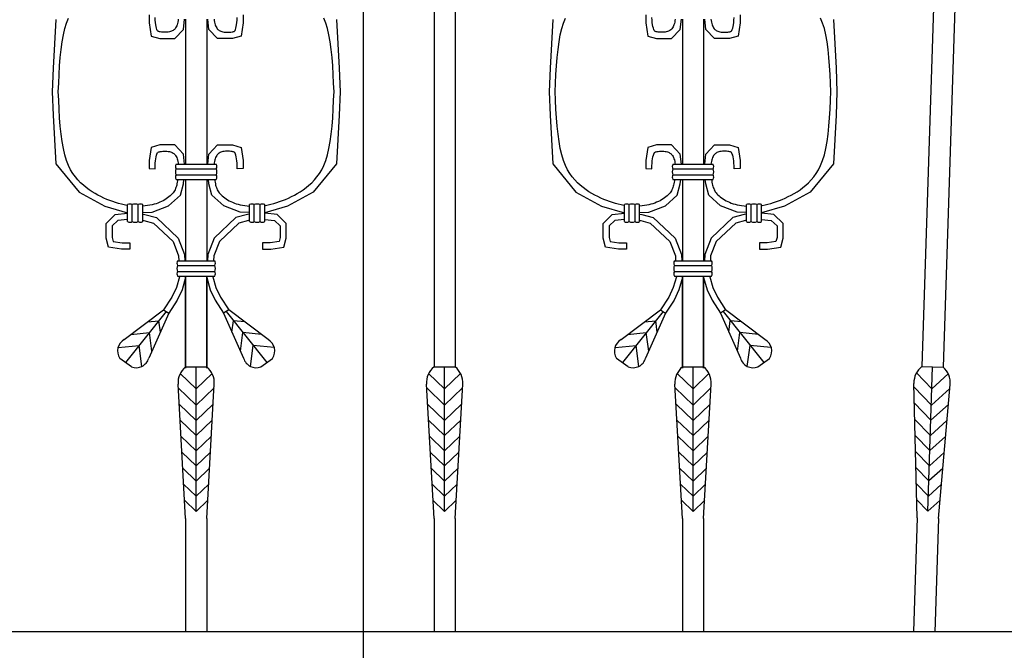
# Model space of a CAD drawing. Units: inches. Extents: x 2278 to 7495, y -71 to 1198.
# Tile 19 of 44: x 5007 to 5033, y 126 to 143. Entities that reach past the tile are written whole.
import ezdxf

# ---------------------------------------------------------------- set-up
doc = ezdxf.new("R2010")
doc.units = ezdxf.units.IN
doc.header["$MEASUREMENT"] = 0
doc.layers.add('A-ANNO-DIMS', color=2, linetype='Continuous', lineweight=18)
doc.layers.add('A-ELEV', color=7, linetype='Continuous', lineweight=25)
doc.styles.get("Standard").update_dxf_attribs({"font": 'arial.ttf'})
doc.dimstyles.get("Standard").update_dxf_attribs({"dimtxt": 6, "dimasz": 3, "dimexe": 0.18, "dimexo": 0.0625, "dimgap": 0.09, "dimtad": 0, "dimtih": 1, "dimtoh": 1, "dimdec": 0, "dimzin": 0, "dimdsep": 46, "dimlunit": 3, "dimtxsty": 'Standard', "dimblk": 'ARCHTICK', "dimcen": 0.09, "dimadec": 0, "dimazin": 0, "dimtfac": 1, "dimtdec": 0, "dimtofl": 0, "dimtmove": 0, "dimatfit": 3, "dimfxl": 1, "dimtolj": 1, "dimtzin": 0, "dimarcsym": 0})

# ---------------------------------------------------------------- blocks, each defined once
blk = doc.blocks.new('BALUSTER-ORNATE-A')
for p, q in [((0.096, 16.469), (0.025, 15.162)), ((0.386, 16.376), (0.438, 16.508)), ((2.602, 16.596), (2.602, 16.378)), ((2.769, 16.452), (2.766, 16.522)), ((2.775, 16.388), (2.769, 16.452)), ((3.383, 16.441), (3.376, 16.401)), ((3.388, 16.479), (3.383, 16.441)), ((3.528, 16.206), (3.557, 16.479)), ((3.585, 16.479), (3.585, 12.578)), ((4.155, 16.479), (4.155, 12.578)), ((4.212, 16.206), (4.183, 16.479)), ((4.352, 16.479), (4.357, 16.441)), ((4.357, 16.441), (4.364, 16.401)), ((4.965, 16.388), (4.971, 16.452)), ((4.971, 16.452), (4.974, 16.522)), ((5.138, 16.596), (5.138, 16.378)), ((7.354, 16.376), (7.302, 16.508)), ((7.644, 16.469), (7.715, 15.162)), ((0.3, 16.057), (0.34, 16.227)), ((0.34, 16.227), (0.386, 16.376)), ((2.602, 16.378), (2.656, 16.024)), ((2.783, 16.331), (2.775, 16.388)), ((2.792, 16.28), (2.783, 16.331)), ((2.803, 16.237), (2.792, 16.28)), ((2.815, 16.203), (2.803, 16.237)), ((2.825, 16.18), (2.815, 16.203)), ((2.834, 16.166), (2.825, 16.18)), ((2.84, 16.159), (2.834, 16.166)), ((2.846, 16.154), (2.84, 16.159)), ((2.852, 16.151), (2.846, 16.154)), ((3.205, 16.154), (3.179, 16.145)), ((3.228, 16.164), (3.205, 16.154)), ((3.249, 16.176), (3.228, 16.164)), ((3.268, 16.19), (3.249, 16.176)), ((3.286, 16.207), (3.268, 16.19)), ((3.303, 16.225), (3.286, 16.207)), ((3.292, 15.961), (3.528, 16.206)), ((3.318, 16.247), (3.303, 16.225)), ((3.333, 16.271), (3.318, 16.247)), ((3.346, 16.299), (3.333, 16.271)), ((3.357, 16.329), (3.346, 16.299)), ((3.368, 16.364), (3.357, 16.329)), ((3.376, 16.401), (3.368, 16.364)), ((4.448, 15.961), (4.212, 16.206)), ((4.364, 16.401), (4.372, 16.364)), ((4.372, 16.364), (4.383, 16.329)), ((4.383, 16.329), (4.394, 16.299)), ((4.394, 16.299), (4.407, 16.271)), ((4.407, 16.271), (4.422, 16.247)), ((4.422, 16.247), (4.437, 16.225)), ((4.437, 16.225), (4.454, 16.207)), ((4.454, 16.207), (4.472, 16.19)), ((4.472, 16.19), (4.491, 16.176)), ((4.491, 16.176), (4.512, 16.164)), ((4.512, 16.164), (4.535, 16.154)), ((4.535, 16.154), (4.561, 16.145)), ((4.888, 16.151), (4.895, 16.154)), ((4.895, 16.154), (4.9, 16.159)), ((4.9, 16.159), (4.906, 16.166)), ((4.906, 16.166), (4.915, 16.18)), ((4.915, 16.18), (4.925, 16.203)), ((4.925, 16.203), (4.937, 16.237)), ((4.937, 16.237), (4.948, 16.28)), ((4.948, 16.28), (4.957, 16.331)), ((4.957, 16.331), (4.965, 16.388)), ((5.138, 16.378), (5.084, 16.024)), ((7.4, 16.227), (7.354, 16.376)), ((7.44, 16.057), (7.4, 16.227)), ((0.267, 15.87), (0.3, 16.057)), ((2.656, 16.024), (2.892, 15.961)), ((2.863, 16.146), (2.852, 16.151)), ((2.88, 16.142), (2.863, 16.146)), ((2.905, 16.137), (2.88, 16.142)), ((2.892, 15.961), (3.292, 15.961)), ((2.936, 16.134), (2.905, 16.137)), ((2.971, 16.131), (2.936, 16.134)), ((3.008, 16.129), (2.971, 16.131)), ((3.045, 16.129), (3.008, 16.129)), ((3.081, 16.13), (3.045, 16.129)), ((3.117, 16.133), (3.081, 16.13)), ((3.15, 16.138), (3.117, 16.133)), ((3.179, 16.145), (3.15, 16.138)), ((4.848, 15.961), (4.448, 15.961)), ((4.561, 16.145), (4.59, 16.138)), ((4.59, 16.138), (4.623, 16.133)), ((4.623, 16.133), (4.659, 16.13)), ((4.659, 16.13), (4.695, 16.129)), ((4.695, 16.129), (4.732, 16.129)), ((4.732, 16.129), (4.769, 16.131)), ((4.769, 16.131), (4.804, 16.134)), ((4.804, 16.134), (4.835, 16.137)), ((4.835, 16.137), (4.86, 16.142)), ((5.084, 16.024), (4.848, 15.961)), ((4.86, 16.142), (4.877, 16.146)), ((4.877, 16.146), (4.888, 16.151)), ((7.473, 15.87), (7.44, 16.057)), ((0.217, 15.452), (0.239, 15.667)), ((0.239, 15.667), (0.267, 15.87)), ((7.501, 15.667), (7.473, 15.87)), ((7.523, 15.452), (7.501, 15.667)), ((0.199, 15.227), (0.217, 15.452)), ((7.541, 15.227), (7.523, 15.452)), ((0.025, 15.162), (0, 14.529)), ((0.185, 14.995), (0.199, 15.227)), ((7.555, 14.995), (7.541, 15.227)), ((7.715, 15.162), (7.74, 14.529)), ((0.173, 14.759), (0.185, 14.995)), ((7.567, 14.759), (7.555, 14.995)), ((0.163, 14.522), (0.173, 14.759)), ((7.577, 14.522), (7.567, 14.759)), ((0, 14.529), (0.025, 13.895)), ((0.173, 14.298), (0.163, 14.536)), ((0.185, 14.062), (0.173, 14.298)), ((7.555, 14.062), (7.567, 14.298)), ((7.567, 14.298), (7.577, 14.536)), ((7.74, 14.529), (7.715, 13.895)), ((0.199, 13.831), (0.185, 14.062)), ((7.541, 13.831), (7.555, 14.062)), ((0.025, 13.895), (0.096, 12.589)), ((0.217, 13.606), (0.199, 13.831)), ((7.523, 13.606), (7.541, 13.831)), ((7.715, 13.895), (7.644, 12.589)), ((0.239, 13.391), (0.217, 13.606)), ((7.501, 13.391), (7.523, 13.606)), ((0.267, 13.188), (0.239, 13.391)), ((7.473, 13.188), (7.501, 13.391)), ((0.3, 13), (0.267, 13.188)), ((0.34, 12.831), (0.3, 13)), ((2.656, 13.033), (2.602, 12.679)), ((2.892, 13.097), (2.656, 13.033)), ((3.292, 13.097), (2.892, 13.097)), ((3.528, 12.852), (3.292, 13.097)), ((4.212, 12.852), (4.448, 13.097)), ((4.448, 13.097), (4.848, 13.097)), ((4.848, 13.097), (5.084, 13.033)), ((5.084, 13.033), (5.138, 12.679)), ((7.4, 12.831), (7.44, 13)), ((7.44, 13), (7.473, 13.188)), ((0.386, 12.681), (0.34, 12.831)), ((2.775, 12.669), (2.783, 12.727)), ((2.783, 12.727), (2.792, 12.778)), ((2.792, 12.778), (2.803, 12.82)), ((2.803, 12.82), (2.815, 12.854)), ((2.815, 12.854), (2.825, 12.878)), ((2.825, 12.878), (2.834, 12.892)), ((2.834, 12.892), (2.84, 12.899)), ((2.84, 12.899), (2.846, 12.903)), ((2.846, 12.903), (2.852, 12.907)), ((2.852, 12.907), (2.863, 12.911)), ((2.863, 12.911), (2.88, 12.916)), ((2.88, 12.916), (2.905, 12.92)), ((2.905, 12.92), (2.936, 12.924)), ((2.936, 12.924), (2.971, 12.927)), ((2.971, 12.927), (3.008, 12.929)), ((3.008, 12.929), (3.045, 12.929)), ((3.045, 12.929), (3.081, 12.928)), ((3.081, 12.928), (3.117, 12.924)), ((3.117, 12.924), (3.15, 12.919)), ((3.15, 12.919), (3.179, 12.912)), ((3.179, 12.912), (3.205, 12.904)), ((3.205, 12.904), (3.228, 12.893)), ((3.228, 12.893), (3.249, 12.881)), ((3.249, 12.881), (3.268, 12.867)), ((3.268, 12.867), (3.286, 12.851)), ((3.286, 12.851), (3.303, 12.832)), ((3.303, 12.832), (3.318, 12.811)), ((3.318, 12.811), (3.333, 12.786)), ((3.333, 12.786), (3.346, 12.759)), ((3.346, 12.759), (3.357, 12.728)), ((3.357, 12.728), (3.368, 12.694)), ((3.557, 12.578), (3.528, 12.852)), ((4.183, 12.578), (4.212, 12.852)), ((4.383, 12.728), (4.372, 12.694)), ((4.394, 12.759), (4.383, 12.728)), ((4.407, 12.786), (4.394, 12.759)), ((4.422, 12.811), (4.407, 12.786)), ((4.437, 12.832), (4.422, 12.811)), ((4.454, 12.851), (4.437, 12.832)), ((4.472, 12.867), (4.454, 12.851)), ((4.491, 12.881), (4.472, 12.867)), ((4.512, 12.893), (4.491, 12.881)), ((4.535, 12.904), (4.512, 12.893)), ((4.561, 12.912), (4.535, 12.904)), ((4.59, 12.919), (4.561, 12.912)), ((4.623, 12.924), (4.59, 12.919)), ((4.659, 12.928), (4.623, 12.924)), ((4.695, 12.929), (4.659, 12.928)), ((4.732, 12.929), (4.695, 12.929)), ((4.769, 12.927), (4.732, 12.929)), ((4.804, 12.924), (4.769, 12.927)), ((4.835, 12.92), (4.804, 12.924)), ((4.86, 12.916), (4.835, 12.92)), ((4.877, 12.911), (4.86, 12.916)), ((4.888, 12.907), (4.877, 12.911)), ((4.895, 12.903), (4.888, 12.907)), ((4.9, 12.899), (4.895, 12.903)), ((4.906, 12.892), (4.9, 12.899)), ((4.915, 12.878), (4.906, 12.892)), ((4.925, 12.854), (4.915, 12.878)), ((4.937, 12.82), (4.925, 12.854)), ((4.948, 12.778), (4.937, 12.82)), ((4.957, 12.727), (4.948, 12.778)), ((4.965, 12.669), (4.957, 12.727)), ((7.354, 12.681), (7.4, 12.831)), ((0.096, 12.589), (0.722, 11.827)), ((0.438, 12.549), (0.386, 12.681)), ((0.495, 12.433), (0.438, 12.549)), ((2.602, 12.679), (2.602, 12.462)), ((2.602, 12.462), (2.764, 12.459)), ((2.764, 12.459), (2.766, 12.536)), ((2.766, 12.536), (2.769, 12.605)), ((2.769, 12.605), (2.775, 12.669)), ((3.329, 12.578), (4.411, 12.578)), ((3.329, 12.456), (4.411, 12.456)), ((3.368, 12.694), (3.376, 12.656)), ((3.376, 12.656), (3.383, 12.616)), ((3.383, 12.616), (3.388, 12.578)), ((4.357, 12.616), (4.352, 12.578)), ((4.364, 12.656), (4.357, 12.616)), ((4.372, 12.694), (4.364, 12.656)), ((4.971, 12.605), (4.965, 12.669)), ((4.974, 12.536), (4.971, 12.605)), ((4.976, 12.459), (4.974, 12.536)), ((5.138, 12.462), (4.976, 12.459)), ((5.138, 12.679), (5.138, 12.462)), ((7.644, 12.589), (7.018, 11.827)), ((7.245, 12.433), (7.302, 12.549)), ((7.302, 12.549), (7.354, 12.681)), ((0.557, 12.33), (0.495, 12.433)), ((0.623, 12.239), (0.557, 12.33)), ((0.692, 12.157), (0.623, 12.239)), ((3.329, 12.293), (4.411, 12.293)), ((7.048, 12.157), (7.117, 12.239)), ((7.117, 12.239), (7.183, 12.33)), ((7.183, 12.33), (7.245, 12.433)), ((0.764, 12.083), (0.692, 12.157)), ((0.839, 12.015), (0.764, 12.083)), ((0.916, 11.952), (0.839, 12.015)), ((0.993, 11.894), (0.916, 11.952)), ((3.316, 11.924), (3.303, 11.895)), ((3.327, 11.954), (3.316, 11.924)), ((3.337, 11.986), (3.327, 11.954)), ((3.329, 12.171), (4.411, 12.171)), ((3.346, 12.02), (3.337, 11.986)), ((3.354, 12.056), (3.346, 12.02)), ((3.361, 12.095), (3.354, 12.056)), ((3.368, 12.136), (3.361, 12.095)), ((3.374, 12.171), (3.368, 12.136)), ((3.446, 11.745), (3.528, 12.053)), ((3.528, 12.053), (3.542, 12.171)), ((3.585, 12.171), (3.585, 9.98)), ((4.155, 12.171), (4.155, 9.98)), ((4.212, 12.053), (4.198, 12.171)), ((4.294, 11.745), (4.212, 12.053)), ((4.366, 12.171), (4.372, 12.136)), ((4.372, 12.136), (4.379, 12.095)), ((4.379, 12.095), (4.386, 12.056)), ((4.386, 12.056), (4.394, 12.02)), ((4.394, 12.02), (4.403, 11.986)), ((4.403, 11.986), (4.413, 11.954)), ((4.413, 11.954), (4.424, 11.924)), ((4.424, 11.924), (4.437, 11.895)), ((6.747, 11.894), (6.824, 11.952)), ((6.824, 11.952), (6.901, 12.015)), ((6.901, 12.015), (6.976, 12.083)), ((6.976, 12.083), (7.048, 12.157)), ((0.722, 11.827), (1.412, 11.455)), ((1.071, 11.841), (0.993, 11.894)), ((1.15, 11.793), (1.071, 11.841)), ((1.23, 11.748), (1.15, 11.793)), ((1.309, 11.708), (1.23, 11.748)), ((1.389, 11.67), (1.309, 11.708)), ((1.469, 11.635), (1.389, 11.67)), ((3.102, 11.673), (3.064, 11.647)), ((3.138, 11.701), (3.102, 11.673)), ((3.128, 11.464), (3.446, 11.745)), ((3.171, 11.729), (3.138, 11.701)), ((3.201, 11.757), (3.171, 11.729)), ((3.228, 11.785), (3.201, 11.757)), ((3.252, 11.813), (3.228, 11.785)), ((3.272, 11.841), (3.252, 11.813)), ((3.288, 11.868), (3.272, 11.841)), ((3.303, 11.895), (3.288, 11.868)), ((4.612, 11.464), (4.294, 11.745)), ((4.437, 11.895), (4.452, 11.868)), ((4.452, 11.868), (4.468, 11.841)), ((4.468, 11.841), (4.489, 11.813)), ((4.489, 11.813), (4.512, 11.785)), ((4.512, 11.785), (4.539, 11.757)), ((4.539, 11.757), (4.569, 11.729)), ((4.569, 11.729), (4.602, 11.701)), ((4.602, 11.701), (4.638, 11.673)), ((4.638, 11.673), (4.676, 11.647)), ((6.271, 11.635), (6.351, 11.67)), ((7.018, 11.827), (6.328, 11.455)), ((6.351, 11.67), (6.431, 11.708)), ((6.431, 11.708), (6.51, 11.748)), ((6.51, 11.748), (6.59, 11.793)), ((6.59, 11.793), (6.669, 11.841)), ((6.669, 11.841), (6.747, 11.894)), ((1.412, 11.455), (2.026, 11.276)), ((1.549, 11.603), (1.469, 11.635)), ((1.627, 11.574), (1.549, 11.603)), ((1.705, 11.548), (1.627, 11.574)), ((1.782, 11.524), (1.705, 11.548)), ((1.858, 11.504), (1.782, 11.524)), ((1.933, 11.487), (1.858, 11.504)), ((2.007, 11.473), (1.933, 11.487)), ((2.026, 11.47), (2.007, 11.473)), ((2.026, 11.037), (2.026, 11.493)), ((2.148, 11.037), (2.148, 11.493)), ((2.311, 11.037), (2.311, 11.493)), ((2.434, 11.037), (2.434, 11.493)), ((2.499, 11.457), (2.434, 11.451)), ((2.563, 11.465), (2.499, 11.457)), ((2.624, 11.476), (2.563, 11.465)), ((2.683, 11.488), (2.624, 11.476)), ((2.739, 11.502), (2.683, 11.488)), ((2.683, 11.291), (3.128, 11.464)), ((2.792, 11.518), (2.739, 11.502)), ((2.843, 11.535), (2.792, 11.518)), ((2.891, 11.555), (2.843, 11.535)), ((2.937, 11.576), (2.891, 11.555)), ((2.981, 11.598), (2.937, 11.576)), ((3.024, 11.622), (2.981, 11.598)), ((3.064, 11.647), (3.024, 11.622)), ((5.057, 11.291), (4.612, 11.464)), ((4.676, 11.647), (4.716, 11.622)), ((4.716, 11.622), (4.759, 11.598)), ((4.759, 11.598), (4.803, 11.576)), ((4.803, 11.576), (4.849, 11.555)), ((4.849, 11.555), (4.897, 11.535)), ((4.897, 11.535), (4.948, 11.518)), ((4.948, 11.518), (5.001, 11.502)), ((5.001, 11.502), (5.057, 11.488)), ((5.057, 11.488), (5.116, 11.476)), ((5.116, 11.476), (5.177, 11.465)), ((5.177, 11.465), (5.241, 11.457)), ((5.241, 11.457), (5.306, 11.451)), ((5.306, 11.037), (5.306, 11.493)), ((5.429, 11.037), (5.429, 11.493)), ((5.592, 11.037), (5.592, 11.493)), ((5.714, 11.037), (5.714, 11.493)), ((5.714, 11.47), (5.733, 11.473)), ((6.328, 11.455), (5.714, 11.276)), ((5.733, 11.473), (5.807, 11.487)), ((5.807, 11.487), (5.882, 11.504)), ((5.882, 11.504), (5.958, 11.524)), ((5.958, 11.524), (6.035, 11.548)), ((6.035, 11.548), (6.113, 11.574)), ((6.113, 11.574), (6.191, 11.603)), ((6.191, 11.603), (6.271, 11.635)), ((1.449, 10.988), (1.694, 11.225)), ((1.694, 11.225), (2.026, 11.261)), ((2.434, 11.28), (2.683, 11.291)), ((2.434, 11.232), (2.492, 11.225)), ((2.492, 11.225), (2.801, 11.143)), ((2.801, 11.143), (3.385, 10.594)), ((4.939, 11.143), (4.355, 10.594)), ((5.248, 11.225), (4.939, 11.143)), ((5.306, 11.28), (5.057, 11.291)), ((5.306, 11.232), (5.248, 11.225)), ((6.046, 11.225), (5.714, 11.261)), ((6.291, 10.988), (6.046, 11.225)), ((1.449, 10.589), (1.449, 10.988)), ((1.767, 11.069), (1.612, 10.919)), ((1.612, 10.919), (1.612, 10.611)), ((2.026, 11.097), (1.767, 11.069)), ((2.434, 11.067), (2.462, 11.064)), ((2.462, 11.064), (2.719, 10.996)), ((2.719, 10.996), (3.247, 10.501)), ((5.021, 10.996), (4.493, 10.501)), ((5.278, 11.064), (5.021, 10.996)), ((5.306, 11.067), (5.278, 11.064)), ((5.714, 11.097), (5.973, 11.069)), ((5.973, 11.069), (6.128, 10.919)), ((6.128, 10.919), (6.128, 10.611)), ((6.291, 10.589), (6.291, 10.988)), ((1.612, 10.611), (1.642, 10.498)), ((3.385, 10.594), (3.558, 10.149)), ((4.355, 10.594), (4.182, 10.149)), ((6.128, 10.611), (6.098, 10.498)), ((1.513, 10.353), (1.449, 10.589)), ((1.866, 10.298), (1.513, 10.353)), ((1.642, 10.498), (1.879, 10.461)), ((1.879, 10.461), (2.084, 10.461)), ((2.084, 10.461), (2.084, 10.298)), ((3.247, 10.501), (3.396, 10.115)), ((4.493, 10.501), (4.344, 10.115)), ((5.861, 10.461), (5.656, 10.461)), ((5.656, 10.461), (5.656, 10.298)), ((6.098, 10.498), (5.861, 10.461)), ((5.874, 10.298), (6.227, 10.353)), ((6.227, 10.353), (6.291, 10.589)), ((2.084, 10.298), (1.866, 10.298)), ((3.396, 10.115), (3.402, 9.98)), ((3.558, 10.149), (3.565, 9.98)), ((4.182, 10.149), (4.175, 9.98)), ((4.344, 10.115), (4.338, 9.98)), ((5.656, 10.298), (5.874, 10.298)), ((3.37, 9.98), (4.37, 9.98)), ((3.37, 9.858), (4.37, 9.858)), ((3.421, 9.552), (3.337, 9.262)), ((3.37, 9.695), (4.37, 9.695)), ((3.37, 9.573), (4.37, 9.573)), ((3.42, 9.573), (3.421, 9.552)), ((3.585, 9.532), (3.49, 9.205)), ((3.583, 9.573), (3.585, 9.532)), ((3.585, 9.573), (3.585, 7.095)), ((3.585, 7.095), (3.585, 9.573)), ((4.155, 9.573), (4.155, 7.095)), ((4.155, 7.095), (4.155, 9.573)), ((4.157, 9.573), (4.155, 9.532)), ((4.155, 9.532), (4.25, 9.205)), ((4.32, 9.573), (4.319, 9.552)), ((4.319, 9.552), (4.403, 9.262)), ((3.337, 9.262), (3.217, 9.001)), ((3.49, 9.205), (3.36, 8.922)), ((4.25, 9.205), (4.38, 8.922)), ((4.403, 9.262), (4.523, 9.001)), ((3.217, 9.001), (2.995, 8.66)), ((3.36, 8.922), (3.131, 8.571)), ((4.38, 8.922), (4.609, 8.571)), ((4.523, 9.001), (4.745, 8.66)), ((1.936, 7.866), (2.995, 8.66)), ((3.063, 8.615), (1.97, 7.244)), ((3.131, 8.571), (2.594, 7.362)), ((2.995, 8.66), (3.131, 8.571)), ((4.745, 8.66), (4.609, 8.571)), ((4.609, 8.571), (5.146, 7.362)), ((4.677, 8.615), (5.77, 7.244)), ((5.804, 7.866), (4.745, 8.66)), ((2.562, 8.34), (2.868, 8.37)), ((2.907, 8.066), (2.868, 8.37)), ((4.833, 8.066), (4.872, 8.37)), ((5.178, 8.34), (4.872, 8.37)), ((2.111, 8.002), (2.613, 8.051)), ((2.678, 7.551), (2.613, 8.051)), ((5.062, 7.551), (5.127, 8.051)), ((5.629, 8.002), (5.127, 8.051)), ((1.774, 7.651), (2.339, 7.706)), ((2.412, 7.143), (2.339, 7.706)), ((5.328, 7.143), (5.401, 7.706)), ((5.966, 7.651), (5.401, 7.706)), ((2.128, 7.128), (1.813, 7.359)), ((5.612, 7.128), (5.927, 7.359)), ((3.442, 6.952), (3.87, 6.538)), ((3.585, 7.128), (4.155, 7.128)), ((3.87, 3.24), (3.87, 7.128)), ((4.299, 6.952), (3.87, 6.538)), ((3.585, 3.055), (3.383, 6.664)), ((4.155, 3.055), (4.357, 6.664)), ((3.388, 6.562), (3.87, 6.097)), ((4.352, 6.562), (3.87, 6.097)), ((3.413, 6.131), (3.87, 5.689)), ((4.327, 6.131), (3.87, 5.689)), ((3.437, 5.699), (3.87, 5.28)), ((4.303, 5.699), (3.87, 5.28)), ((3.461, 5.268), (3.87, 4.872)), ((4.279, 5.268), (3.87, 4.872)), ((3.485, 4.836), (3.87, 4.464)), ((4.255, 4.836), (3.87, 4.464)), ((3.509, 4.405), (3.87, 4.056)), ((4.231, 4.405), (3.87, 4.056)), ((3.533, 3.973), (3.87, 3.648)), ((4.207, 3.973), (3.87, 3.648)), ((3.558, 3.542), (3.87, 3.24)), ((4.182, 3.542), (3.87, 3.24)), ((3.585, 3.055), (3.585, 0)), ((4.155, 3.055), (4.155, 0))]:
    blk.add_line(p, q)
for centre, radius, start, end in [((3.434, 12.517), 0.121, 149.7768, 210.2232), ((3.522, 12.375), 0.209, 157.1017, 202.8983), ((4.306, 12.517), 0.121, 329.7768, 30.2232), ((4.218, 12.375), 0.209, 337.1017, 22.8983), ((3.434, 12.232), 0.121, 149.7768, 210.2232), ((4.306, 12.232), 0.121, 329.7768, 30.2232), ((2.087, 11.388), 0.121, 59.7768, 120.2232), ((2.23, 11.3), 0.209, 67.1017, 112.8983), ((2.373, 11.388), 0.121, 59.7768, 120.2232), ((5.368, 11.388), 0.121, 59.7768, 120.2232), ((5.51, 11.3), 0.209, 67.1017, 112.8983), ((5.653, 11.388), 0.121, 59.7768, 120.2232), ((2.087, 11.142), 0.121, 239.7768, 300.2232), ((2.23, 11.23), 0.209, 247.1017, 292.8983), ((2.373, 11.142), 0.121, 239.7768, 300.2232), ((5.368, 11.142), 0.121, 239.7768, 300.2232), ((5.51, 11.23), 0.209, 247.1017, 292.8983), ((5.653, 11.142), 0.121, 239.7768, 300.2232), ((3.475, 9.919), 0.121, 149.7768, 210.2232), ((3.563, 9.776), 0.209, 157.1017, 202.8983), ((4.265, 9.919), 0.121, 329.7768, 30.2232), ((4.177, 9.776), 0.209, 337.1017, 22.8983), ((3.475, 9.634), 0.121, 149.7768, 210.2232), ((4.265, 9.634), 0.121, 329.7768, 30.2232), ((2.111, 7.555), 0.356, 119.3212, 213.425), ((5.629, 7.555), 0.356, 326.575, 60.6788), ((2.253, 7.462), 0.356, 249.4937, 343.5975), ((5.487, 7.462), 0.356, 196.4025, 290.5063), ((3.929, 6.703), 0.547, 128.9283, 183.9822), ((3.811, 6.703), 0.547, 356.0178, 51.0717)]:
    blk.add_arc(centre, radius, start, end)
blk = doc.blocks.new('BALUSTER-ORNATE-B')
for p, q in [((0.096, 16.469), (0.025, 15.162)), ((0.386, 16.376), (0.438, 16.508)), ((2.602, 16.596), (2.602, 16.378)), ((2.769, 16.452), (2.766, 16.522)), ((2.775, 16.388), (2.769, 16.452)), ((3.384, 16.441), (3.377, 16.401)), ((3.388, 16.479), (3.384, 16.441)), ((3.528, 16.206), (3.558, 16.479)), ((3.585, 16.479), (3.585, 12.578)), ((4.155, 16.479), (4.155, 12.578)), ((4.213, 16.206), (4.183, 16.479)), ((4.352, 16.479), (4.357, 16.441)), ((4.357, 16.441), (4.364, 16.401)), ((4.965, 16.388), (4.971, 16.452)), ((4.971, 16.452), (4.975, 16.522)), ((5.139, 16.596), (5.139, 16.378)), ((7.354, 16.376), (7.302, 16.508)), ((7.645, 16.469), (7.715, 15.162)), ((0.3, 16.057), (0.34, 16.227)), ((0.34, 16.227), (0.386, 16.376)), ((2.602, 16.378), (2.656, 16.024)), ((2.783, 16.331), (2.775, 16.388)), ((2.793, 16.28), (2.783, 16.331)), ((2.803, 16.237), (2.793, 16.28)), ((2.815, 16.203), (2.803, 16.237)), ((2.826, 16.18), (2.815, 16.203)), ((2.834, 16.166), (2.826, 16.18)), ((2.841, 16.159), (2.834, 16.166)), ((2.846, 16.154), (2.841, 16.159)), ((2.852, 16.151), (2.846, 16.154)), ((3.206, 16.154), (3.18, 16.145)), ((3.229, 16.164), (3.206, 16.154)), ((3.249, 16.176), (3.229, 16.164)), ((3.269, 16.19), (3.249, 16.176)), ((3.286, 16.207), (3.269, 16.19)), ((3.303, 16.225), (3.286, 16.207)), ((3.292, 15.961), (3.528, 16.206)), ((3.319, 16.247), (3.303, 16.225)), ((3.333, 16.271), (3.319, 16.247)), ((3.346, 16.299), (3.333, 16.271)), ((3.358, 16.329), (3.346, 16.299)), ((3.368, 16.364), (3.358, 16.329)), ((3.377, 16.401), (3.368, 16.364)), ((4.449, 15.961), (4.213, 16.206)), ((4.364, 16.401), (4.373, 16.364)), ((4.373, 16.364), (4.383, 16.329)), ((4.383, 16.329), (4.394, 16.299)), ((4.394, 16.299), (4.407, 16.271)), ((4.407, 16.271), (4.422, 16.247)), ((4.422, 16.247), (4.437, 16.225)), ((4.437, 16.225), (4.454, 16.207)), ((4.454, 16.207), (4.472, 16.19)), ((4.472, 16.19), (4.491, 16.176)), ((4.491, 16.176), (4.512, 16.164)), ((4.512, 16.164), (4.535, 16.154)), ((4.535, 16.154), (4.561, 16.145)), ((4.888, 16.151), (4.895, 16.154)), ((4.895, 16.154), (4.9, 16.159)), ((4.9, 16.159), (4.906, 16.166)), ((4.906, 16.166), (4.915, 16.18)), ((4.915, 16.18), (4.926, 16.203)), ((4.926, 16.203), (4.937, 16.237)), ((4.937, 16.237), (4.948, 16.28)), ((4.948, 16.28), (4.958, 16.331)), ((4.958, 16.331), (4.965, 16.388)), ((5.139, 16.378), (5.084, 16.024)), ((7.401, 16.227), (7.354, 16.376)), ((7.44, 16.057), (7.401, 16.227)), ((0.267, 15.87), (0.3, 16.057)), ((2.656, 16.024), (2.892, 15.961)), ((2.863, 16.146), (2.852, 16.151)), ((2.881, 16.142), (2.863, 16.146)), ((2.905, 16.137), (2.881, 16.142)), ((2.892, 15.961), (3.292, 15.961)), ((2.936, 16.134), (2.905, 16.137)), ((2.971, 16.131), (2.936, 16.134)), ((3.008, 16.129), (2.971, 16.131)), ((3.045, 16.129), (3.008, 16.129)), ((3.082, 16.13), (3.045, 16.129)), ((3.117, 16.133), (3.082, 16.13)), ((3.15, 16.138), (3.117, 16.133)), ((3.18, 16.145), (3.15, 16.138)), ((4.848, 15.961), (4.449, 15.961)), ((4.561, 16.145), (4.591, 16.138)), ((4.591, 16.138), (4.624, 16.133)), ((4.624, 16.133), (4.659, 16.13)), ((4.659, 16.13), (4.696, 16.129)), ((4.696, 16.129), (4.733, 16.129)), ((4.733, 16.129), (4.769, 16.131)), ((4.769, 16.131), (4.805, 16.134)), ((4.805, 16.134), (4.836, 16.137)), ((4.836, 16.137), (4.86, 16.142)), ((5.084, 16.024), (4.848, 15.961)), ((4.86, 16.142), (4.877, 16.146)), ((4.877, 16.146), (4.888, 16.151)), ((7.473, 15.87), (7.44, 16.057)), ((0.217, 15.452), (0.24, 15.667)), ((0.24, 15.667), (0.267, 15.87)), ((7.501, 15.667), (7.473, 15.87)), ((7.523, 15.452), (7.501, 15.667)), ((0.199, 15.227), (0.217, 15.452)), ((7.541, 15.227), (7.523, 15.452)), ((0.025, 15.162), (0, 14.529)), ((0.185, 14.995), (0.199, 15.227)), ((7.556, 14.995), (7.541, 15.227)), ((7.715, 15.162), (7.74, 14.529)), ((0.173, 14.759), (0.185, 14.995)), ((7.567, 14.759), (7.556, 14.995)), ((0.163, 14.522), (0.173, 14.759)), ((7.577, 14.522), (7.567, 14.759)), ((0, 14.529), (0.025, 13.895)), ((0.173, 14.298), (0.163, 14.536)), ((0.185, 14.062), (0.173, 14.298)), ((7.556, 14.062), (7.567, 14.298)), ((7.567, 14.298), (7.577, 14.536)), ((7.74, 14.529), (7.715, 13.895)), ((0.199, 13.831), (0.185, 14.062)), ((7.541, 13.831), (7.556, 14.062)), ((0.025, 13.895), (0.096, 12.589)), ((0.217, 13.606), (0.199, 13.831)), ((7.523, 13.606), (7.541, 13.831)), ((7.715, 13.895), (7.645, 12.589)), ((0.24, 13.391), (0.217, 13.606)), ((7.501, 13.391), (7.523, 13.606)), ((0.267, 13.188), (0.24, 13.391)), ((7.473, 13.188), (7.501, 13.391)), ((0.3, 13), (0.267, 13.188)), ((0.34, 12.831), (0.3, 13)), ((2.656, 13.033), (2.602, 12.679)), ((2.892, 13.097), (2.656, 13.033)), ((3.292, 13.097), (2.892, 13.097)), ((3.528, 12.852), (3.292, 13.097)), ((4.213, 12.852), (4.449, 13.097)), ((4.449, 13.097), (4.848, 13.097)), ((4.848, 13.097), (5.084, 13.033)), ((5.084, 13.033), (5.139, 12.679)), ((7.401, 12.831), (7.44, 13)), ((7.44, 13), (7.473, 13.188)), ((0.386, 12.681), (0.34, 12.831)), ((2.775, 12.669), (2.783, 12.727)), ((2.783, 12.727), (2.793, 12.778)), ((2.793, 12.778), (2.803, 12.82)), ((2.803, 12.82), (2.815, 12.854)), ((2.815, 12.854), (2.826, 12.878)), ((2.826, 12.878), (2.834, 12.892)), ((2.834, 12.892), (2.841, 12.899)), ((2.841, 12.899), (2.846, 12.903)), ((2.846, 12.903), (2.852, 12.907)), ((2.852, 12.907), (2.863, 12.911)), ((2.863, 12.911), (2.881, 12.916)), ((2.881, 12.916), (2.905, 12.92)), ((2.905, 12.92), (2.936, 12.924)), ((2.936, 12.924), (2.971, 12.927)), ((2.971, 12.927), (3.008, 12.929)), ((3.008, 12.929), (3.045, 12.929)), ((3.045, 12.929), (3.082, 12.928)), ((3.082, 12.928), (3.117, 12.924)), ((3.117, 12.924), (3.15, 12.919)), ((3.15, 12.919), (3.18, 12.912)), ((3.18, 12.912), (3.206, 12.904)), ((3.206, 12.904), (3.229, 12.893)), ((3.229, 12.893), (3.249, 12.881)), ((3.249, 12.881), (3.269, 12.867)), ((3.269, 12.867), (3.286, 12.851)), ((3.286, 12.851), (3.303, 12.832)), ((3.303, 12.832), (3.319, 12.811)), ((3.319, 12.811), (3.333, 12.786)), ((3.333, 12.786), (3.346, 12.759)), ((3.346, 12.759), (3.358, 12.728)), ((3.358, 12.728), (3.368, 12.694)), ((3.558, 12.578), (3.528, 12.852)), ((4.183, 12.578), (4.213, 12.852)), ((4.383, 12.728), (4.373, 12.694)), ((4.394, 12.759), (4.383, 12.728)), ((4.407, 12.786), (4.394, 12.759)), ((4.422, 12.811), (4.407, 12.786)), ((4.437, 12.832), (4.422, 12.811)), ((4.454, 12.851), (4.437, 12.832)), ((4.472, 12.867), (4.454, 12.851)), ((4.491, 12.881), (4.472, 12.867)), ((4.512, 12.893), (4.491, 12.881)), ((4.535, 12.904), (4.512, 12.893)), ((4.561, 12.912), (4.535, 12.904)), ((4.591, 12.919), (4.561, 12.912)), ((4.624, 12.924), (4.591, 12.919)), ((4.659, 12.928), (4.624, 12.924)), ((4.696, 12.929), (4.659, 12.928)), ((4.733, 12.929), (4.696, 12.929)), ((4.769, 12.927), (4.733, 12.929)), ((4.805, 12.924), (4.769, 12.927)), ((4.836, 12.92), (4.805, 12.924)), ((4.86, 12.916), (4.836, 12.92)), ((4.877, 12.911), (4.86, 12.916)), ((4.888, 12.907), (4.877, 12.911)), ((4.895, 12.903), (4.888, 12.907)), ((4.9, 12.899), (4.895, 12.903)), ((4.906, 12.892), (4.9, 12.899)), ((4.915, 12.878), (4.906, 12.892)), ((4.926, 12.854), (4.915, 12.878)), ((4.937, 12.82), (4.926, 12.854)), ((4.948, 12.778), (4.937, 12.82)), ((4.958, 12.727), (4.948, 12.778)), ((4.965, 12.669), (4.958, 12.727)), ((7.354, 12.681), (7.401, 12.831)), ((0.096, 12.589), (0.722, 11.827)), ((0.438, 12.549), (0.386, 12.681)), ((0.496, 12.433), (0.438, 12.549)), ((2.602, 12.679), (2.602, 12.462)), ((2.602, 12.462), (2.765, 12.459)), ((2.765, 12.459), (2.766, 12.536)), ((2.766, 12.536), (2.769, 12.605)), ((2.769, 12.605), (2.775, 12.669)), ((3.33, 12.578), (4.411, 12.578)), ((3.33, 12.456), (4.411, 12.456)), ((3.368, 12.694), (3.377, 12.656)), ((3.377, 12.656), (3.384, 12.616)), ((3.384, 12.616), (3.388, 12.578)), ((4.357, 12.616), (4.352, 12.578)), ((4.364, 12.656), (4.357, 12.616)), ((4.373, 12.694), (4.364, 12.656)), ((4.971, 12.605), (4.965, 12.669)), ((4.975, 12.536), (4.971, 12.605)), ((4.976, 12.459), (4.975, 12.536)), ((5.139, 12.462), (4.976, 12.459)), ((5.139, 12.679), (5.139, 12.462)), ((7.645, 12.589), (7.018, 11.827)), ((7.245, 12.433), (7.302, 12.549)), ((7.302, 12.549), (7.354, 12.681)), ((0.557, 12.33), (0.496, 12.433)), ((0.623, 12.239), (0.557, 12.33)), ((0.692, 12.157), (0.623, 12.239)), ((3.33, 12.293), (4.411, 12.293)), ((7.048, 12.157), (7.117, 12.239)), ((7.117, 12.239), (7.183, 12.33)), ((7.183, 12.33), (7.245, 12.433)), ((0.765, 12.083), (0.692, 12.157)), ((0.839, 12.015), (0.765, 12.083)), ((0.916, 11.952), (0.839, 12.015)), ((0.994, 11.894), (0.916, 11.952)), ((3.316, 11.924), (3.303, 11.895)), ((3.327, 11.954), (3.316, 11.924)), ((3.337, 11.986), (3.327, 11.954)), ((3.33, 12.171), (4.411, 12.171)), ((3.346, 12.02), (3.337, 11.986)), ((3.354, 12.056), (3.346, 12.02)), ((3.362, 12.095), (3.354, 12.056)), ((3.369, 12.136), (3.362, 12.095)), ((3.374, 12.171), (3.369, 12.136)), ((3.446, 11.745), (3.528, 12.053)), ((3.528, 12.053), (3.542, 12.171)), ((3.585, 12.171), (3.585, 9.98)), ((4.155, 12.171), (4.155, 9.98)), ((4.213, 12.053), (4.199, 12.171)), ((4.294, 11.745), (4.213, 12.053)), ((4.366, 12.171), (4.372, 12.136)), ((4.372, 12.136), (4.379, 12.095)), ((4.379, 12.095), (4.387, 12.056)), ((4.387, 12.056), (4.395, 12.02)), ((4.395, 12.02), (4.404, 11.986)), ((4.404, 11.986), (4.413, 11.954)), ((4.413, 11.954), (4.425, 11.924)), ((4.425, 11.924), (4.437, 11.895)), ((6.747, 11.894), (6.825, 11.952)), ((6.825, 11.952), (6.901, 12.015)), ((6.901, 12.015), (6.976, 12.083)), ((6.976, 12.083), (7.048, 12.157)), ((0.722, 11.827), (1.412, 11.455)), ((1.072, 11.841), (0.994, 11.894)), ((1.151, 11.793), (1.072, 11.841)), ((1.23, 11.748), (1.151, 11.793)), ((1.309, 11.708), (1.23, 11.748)), ((1.389, 11.67), (1.309, 11.708)), ((1.469, 11.635), (1.389, 11.67)), ((3.103, 11.673), (3.064, 11.647)), ((3.138, 11.701), (3.103, 11.673)), ((3.128, 11.464), (3.446, 11.745)), ((3.171, 11.729), (3.138, 11.701)), ((3.201, 11.757), (3.171, 11.729)), ((3.228, 11.785), (3.201, 11.757)), ((3.252, 11.813), (3.228, 11.785)), ((3.272, 11.841), (3.252, 11.813)), ((3.289, 11.868), (3.272, 11.841)), ((3.303, 11.895), (3.289, 11.868)), ((4.612, 11.464), (4.294, 11.745)), ((4.437, 11.895), (4.452, 11.868)), ((4.452, 11.868), (4.469, 11.841)), ((4.469, 11.841), (4.489, 11.813)), ((4.489, 11.813), (4.512, 11.785)), ((4.512, 11.785), (4.539, 11.757)), ((4.539, 11.757), (4.569, 11.729)), ((4.569, 11.729), (4.602, 11.701)), ((4.602, 11.701), (4.638, 11.673)), ((4.638, 11.673), (4.676, 11.647)), ((6.271, 11.635), (6.351, 11.67)), ((7.018, 11.827), (6.328, 11.455)), ((6.351, 11.67), (6.431, 11.708)), ((6.431, 11.708), (6.511, 11.748)), ((6.511, 11.748), (6.59, 11.793)), ((6.59, 11.793), (6.669, 11.841)), ((6.669, 11.841), (6.747, 11.894)), ((1.412, 11.455), (2.027, 11.276)), ((1.549, 11.603), (1.469, 11.635)), ((1.628, 11.574), (1.549, 11.603)), ((1.705, 11.548), (1.628, 11.574)), ((1.782, 11.524), (1.705, 11.548)), ((1.858, 11.504), (1.782, 11.524)), ((1.933, 11.487), (1.858, 11.504)), ((2.008, 11.473), (1.933, 11.487)), ((2.027, 11.47), (2.008, 11.473)), ((2.027, 11.037), (2.027, 11.493)), ((2.149, 11.037), (2.149, 11.493)), ((2.312, 11.037), (2.312, 11.493)), ((2.434, 11.037), (2.434, 11.493)), ((2.5, 11.457), (2.434, 11.451)), ((2.563, 11.465), (2.5, 11.457)), ((2.625, 11.476), (2.563, 11.465)), ((2.683, 11.488), (2.625, 11.476)), ((2.739, 11.502), (2.683, 11.488)), ((2.684, 11.291), (3.128, 11.464)), ((2.792, 11.518), (2.739, 11.502)), ((2.843, 11.535), (2.792, 11.518)), ((2.891, 11.555), (2.843, 11.535)), ((2.937, 11.576), (2.891, 11.555)), ((2.982, 11.598), (2.937, 11.576)), ((3.024, 11.622), (2.982, 11.598)), ((3.064, 11.647), (3.024, 11.622)), ((5.057, 11.291), (4.612, 11.464)), ((4.676, 11.647), (4.717, 11.622)), ((4.717, 11.622), (4.759, 11.598)), ((4.759, 11.598), (4.803, 11.576)), ((4.803, 11.576), (4.849, 11.555)), ((4.849, 11.555), (4.898, 11.535)), ((4.898, 11.535), (4.948, 11.518)), ((4.948, 11.518), (5.002, 11.502)), ((5.002, 11.502), (5.057, 11.488)), ((5.057, 11.488), (5.116, 11.476)), ((5.116, 11.476), (5.177, 11.465)), ((5.177, 11.465), (5.241, 11.457)), ((5.241, 11.457), (5.307, 11.451)), ((5.307, 11.037), (5.307, 11.493)), ((5.429, 11.037), (5.429, 11.493)), ((5.592, 11.037), (5.592, 11.493)), ((5.714, 11.037), (5.714, 11.493)), ((5.714, 11.47), (5.733, 11.473)), ((6.328, 11.455), (5.714, 11.276)), ((5.733, 11.473), (5.807, 11.487)), ((5.807, 11.487), (5.882, 11.504)), ((5.882, 11.504), (5.958, 11.524)), ((5.958, 11.524), (6.035, 11.548)), ((6.035, 11.548), (6.113, 11.574)), ((6.113, 11.574), (6.192, 11.603)), ((6.192, 11.603), (6.271, 11.635)), ((1.449, 10.988), (1.694, 11.225)), ((1.694, 11.225), (2.027, 11.261)), ((2.434, 11.28), (2.684, 11.291)), ((2.434, 11.232), (2.493, 11.225)), ((2.493, 11.225), (2.801, 11.143)), ((2.801, 11.143), (3.386, 10.594)), ((4.939, 11.143), (4.355, 10.594)), ((5.248, 11.225), (4.939, 11.143)), ((5.307, 11.28), (5.057, 11.291)), ((5.307, 11.232), (5.248, 11.225)), ((6.046, 11.225), (5.714, 11.261)), ((6.291, 10.988), (6.046, 11.225)), ((1.449, 10.589), (1.449, 10.988)), ((1.767, 11.069), (1.612, 10.919)), ((1.612, 10.919), (1.612, 10.611)), ((2.027, 11.097), (1.767, 11.069)), ((2.434, 11.067), (2.462, 11.064)), ((2.462, 11.064), (2.72, 10.996)), ((2.72, 10.996), (3.247, 10.501)), ((5.021, 10.996), (4.494, 10.501)), ((5.279, 11.064), (5.021, 10.996)), ((5.307, 11.067), (5.279, 11.064)), ((5.714, 11.097), (5.973, 11.069)), ((5.973, 11.069), (6.128, 10.919)), ((6.128, 10.919), (6.128, 10.611)), ((6.291, 10.589), (6.291, 10.988)), ((1.612, 10.611), (1.643, 10.498)), ((3.386, 10.594), (3.558, 10.149)), ((4.355, 10.594), (4.183, 10.149)), ((6.128, 10.611), (6.098, 10.498)), ((1.513, 10.353), (1.449, 10.589)), ((1.867, 10.298), (1.513, 10.353)), ((1.643, 10.498), (1.879, 10.461)), ((1.879, 10.461), (2.084, 10.461)), ((2.084, 10.461), (2.084, 10.298)), ((3.247, 10.501), (3.396, 10.115)), ((4.494, 10.501), (4.344, 10.115)), ((5.861, 10.461), (5.656, 10.461)), ((5.656, 10.461), (5.656, 10.298)), ((6.098, 10.498), (5.861, 10.461)), ((5.874, 10.298), (6.228, 10.353)), ((6.228, 10.353), (6.291, 10.589)), ((2.084, 10.298), (1.867, 10.298)), ((3.396, 10.115), (3.402, 9.98)), ((3.558, 10.149), (3.565, 9.98)), ((4.183, 10.149), (4.175, 9.98)), ((4.344, 10.115), (4.338, 9.98)), ((5.656, 10.298), (5.874, 10.298)), ((3.37, 9.98), (4.37, 9.98)), ((3.37, 9.858), (4.37, 9.858)), ((3.421, 9.552), (3.337, 9.262)), ((3.37, 9.695), (4.37, 9.695)), ((3.37, 9.573), (4.37, 9.573)), ((3.42, 9.573), (3.421, 9.552)), ((3.585, 9.532), (3.49, 9.205)), ((3.583, 9.573), (3.585, 9.532)), ((3.585, 9.573), (3.585, 7.095)), ((3.585, 7.095), (3.585, 9.573)), ((4.155, 9.573), (4.155, 7.095)), ((4.155, 7.095), (4.155, 9.573)), ((4.157, 9.573), (4.155, 9.532)), ((4.155, 9.532), (4.251, 9.205)), ((4.32, 9.573), (4.319, 9.552)), ((4.319, 9.552), (4.404, 9.262)), ((3.337, 9.262), (3.217, 9.001)), ((3.49, 9.205), (3.36, 8.922)), ((4.251, 9.205), (4.381, 8.922)), ((4.404, 9.262), (4.524, 9.001)), ((3.217, 9.001), (2.995, 8.66)), ((3.36, 8.922), (3.132, 8.571)), ((4.381, 8.922), (4.609, 8.571)), ((4.524, 9.001), (4.746, 8.66)), ((1.936, 7.866), (2.995, 8.66)), ((3.063, 8.615), (1.971, 7.244)), ((3.132, 8.571), (2.595, 7.362)), ((2.995, 8.66), (3.132, 8.571)), ((4.746, 8.66), (4.609, 8.571)), ((4.609, 8.571), (5.146, 7.362)), ((4.677, 8.615), (5.77, 7.244)), ((5.804, 7.866), (4.746, 8.66)), ((2.563, 8.34), (2.868, 8.37)), ((2.907, 8.066), (2.868, 8.37)), ((4.833, 8.066), (4.873, 8.37)), ((5.178, 8.34), (4.873, 8.37)), ((2.112, 8.002), (2.614, 8.051)), ((2.679, 7.551), (2.614, 8.051)), ((5.062, 7.551), (5.127, 8.051)), ((5.629, 8.002), (5.127, 8.051)), ((1.774, 7.651), (2.339, 7.706)), ((2.412, 7.143), (2.339, 7.706)), ((5.328, 7.143), (5.402, 7.706)), ((5.966, 7.651), (5.402, 7.706)), ((2.128, 7.128), (1.814, 7.359)), ((5.613, 7.128), (5.927, 7.359)), ((3.442, 6.952), (3.87, 6.538)), ((3.585, 7.128), (4.155, 7.128)), ((3.87, 3.24), (3.87, 7.128)), ((4.299, 6.952), (3.87, 6.538)), ((3.585, 3.055), (3.383, 6.664)), ((4.155, 3.055), (4.358, 6.664)), ((3.389, 6.562), (3.87, 6.097)), ((4.352, 6.562), (3.87, 6.097)), ((3.413, 6.131), (3.87, 5.689)), ((4.328, 6.131), (3.87, 5.689)), ((3.437, 5.699), (3.87, 5.28)), ((4.304, 5.699), (3.87, 5.28)), ((3.461, 5.268), (3.87, 4.872)), ((4.279, 5.268), (3.87, 4.872)), ((3.485, 4.836), (3.87, 4.464)), ((4.255, 4.836), (3.87, 4.464)), ((3.51, 4.405), (3.87, 4.056)), ((4.231, 4.405), (3.87, 4.056)), ((3.534, 3.973), (3.87, 3.648)), ((4.207, 3.973), (3.87, 3.648)), ((3.558, 3.542), (3.87, 3.24)), ((4.183, 3.542), (3.87, 3.24)), ((3.585, 3.055), (3.585, 0)), ((4.155, 3.055), (4.155, 0))]:
    blk.add_line(p, q)
for centre, radius, start, end in [((3.434, 12.517), 0.121, 149.7768, 210.2232), ((3.522, 12.375), 0.209, 157.1017, 202.8983), ((4.306, 12.517), 0.121, 329.7768, 30.2232), ((4.218, 12.375), 0.209, 337.1017, 22.8983), ((3.434, 12.232), 0.121, 149.7768, 210.2232), ((4.306, 12.232), 0.121, 329.7768, 30.2232), ((2.088, 11.388), 0.121, 59.7768, 120.2232), ((2.23, 11.3), 0.209, 67.1017, 112.8983), ((2.373, 11.388), 0.121, 59.7768, 120.2232), ((5.368, 11.388), 0.121, 59.7768, 120.2232), ((5.51, 11.3), 0.209, 67.1017, 112.8983), ((5.653, 11.388), 0.121, 59.7768, 120.2232), ((2.088, 11.142), 0.121, 239.7768, 300.2232), ((2.23, 11.23), 0.209, 247.1017, 292.8983), ((2.373, 11.142), 0.121, 239.7768, 300.2232), ((5.368, 11.142), 0.121, 239.7768, 300.2232), ((5.51, 11.23), 0.209, 247.1017, 292.8983), ((5.653, 11.142), 0.121, 239.7768, 300.2232), ((3.475, 9.919), 0.121, 149.7768, 210.2232), ((3.563, 9.776), 0.209, 157.1017, 202.8983), ((4.265, 9.919), 0.121, 329.7768, 30.2232), ((4.177, 9.776), 0.209, 337.1017, 22.8983), ((3.475, 9.634), 0.121, 149.7768, 210.2232), ((4.265, 9.634), 0.121, 329.7768, 30.2232), ((2.111, 7.555), 0.356, 119.3212, 213.425), ((5.63, 7.555), 0.356, 326.575, 60.6788), ((2.253, 7.462), 0.356, 249.4937, 343.5975), ((5.488, 7.462), 0.356, 196.4025, 290.5063), ((3.929, 6.703), 0.547, 128.9283, 183.9822), ((3.811, 6.703), 0.547, 356.0178, 51.0717)]:
    blk.add_arc(centre, radius, start, end)
blk = doc.blocks.new('RAIL-BAR-A')
for p, q in [((0.202, 21.929), (0.202, 7.128)), ((0.773, 21.929), (0.773, 7.128)), ((0.059, 6.952), (0.488, 6.538)), ((0.202, 7.128), (0.773, 7.128)), ((0.488, 3.24), (0.488, 7.128)), ((0.916, 6.952), (0.488, 6.538)), ((0.202, 3.055), (0, 6.664)), ((0.773, 3.055), (0.975, 6.664)), ((0.006, 6.562), (0.488, 6.097)), ((0.969, 6.562), (0.488, 6.097)), ((0.03, 6.131), (0.488, 5.689)), ((0.945, 6.131), (0.488, 5.689)), ((0.054, 5.699), (0.488, 5.28)), ((0.921, 5.699), (0.488, 5.28)), ((0.079, 5.268), (0.488, 4.872)), ((0.897, 5.268), (0.488, 4.872)), ((0.103, 4.836), (0.488, 4.464)), ((0.873, 4.836), (0.488, 4.464)), ((0.127, 4.405), (0.488, 4.056)), ((0.848, 4.405), (0.488, 4.056)), ((0.151, 3.973), (0.488, 3.648)), ((0.824, 3.973), (0.488, 3.648)), ((0.175, 3.542), (0.488, 3.24)), ((0.8, 3.542), (0.488, 3.24)), ((0.202, 3.055), (0.202, 0)), ((0.773, 3.055), (0.773, 0))]:
    blk.add_line(p, q)
for centre, start, end in [((0.546, 6.703), 128.9283, 183.9822), ((0.429, 6.703), 356.0178, 51.0717)]:
    blk.add_arc(centre, 0.547, start, end)
blk = doc.blocks.new('RAIL-BAR-C')
for p, q in [((0.203, 21.929), (0.203, 7.128)), ((0.773, 21.929), (0.773, 7.128)), ((0.059, 6.952), (0.488, 6.538)), ((0.203, 7.128), (0.773, 7.128)), ((0.488, 3.24), (0.488, 7.128)), ((0.916, 6.952), (0.488, 6.538)), ((0.203, 3.055), (0, 6.664)), ((0.773, 3.055), (0.975, 6.664)), ((0.006, 6.562), (0.488, 6.097)), ((0.969, 6.562), (0.488, 6.097)), ((0.03, 6.131), (0.488, 5.689)), ((0.945, 6.131), (0.488, 5.689)), ((0.054, 5.699), (0.488, 5.28)), ((0.921, 5.699), (0.488, 5.28)), ((0.079, 5.268), (0.488, 4.872)), ((0.897, 5.268), (0.488, 4.872)), ((0.103, 4.836), (0.488, 4.464)), ((0.873, 4.836), (0.488, 4.464)), ((0.127, 4.405), (0.488, 4.056)), ((0.848, 4.405), (0.488, 4.056)), ((0.151, 3.973), (0.488, 3.648)), ((0.824, 3.973), (0.488, 3.648)), ((0.175, 3.542), (0.488, 3.24)), ((0.8, 3.542), (0.488, 3.24)), ((0.203, 3.055), (0.203, 0)), ((0.773, 3.055), (0.773, 0))]:
    blk.add_line(p, q)
for centre, start, end in [((0.547, 6.703), 128.9283, 183.9822), ((0.429, 6.703), 356.0178, 51.0717)]:
    blk.add_arc(centre, 0.547, start, end)
blk = doc.blocks.new('_ArchTick')
at = {"color": 0, "linetype": 'ByBlock', "const_width": 0.15}
blk.add_lwpolyline([(-0.5, -0.5), (0.5, 0.5)], dxfattribs=at)
blk = doc.blocks.new('*D123')
at = {"layer": 'A-ANNO-DIMS', "color": 0, "lineweight": -2, "transparency": 16777216}
for p, q in [((4736.95, 340.157), (4736.95, -23.427)), ((5145.676, -1.81), (5145.676, -23.427)), ((4736.95, -23.247), (4923.929, -23.247)), ((5145.676, -23.247), (4958.697, -23.247))]:
    blk.add_line(p, q, dxfattribs=at)
at = {"layer": 'Defpoints', "color": 0, "transparency": 16777216}
for p in [(4736.95, 340.219), (5145.676, -1.747), (5145.676, -23.247)]:
    blk.add_point(p, dxfattribs=at)
at = {"layer": 'A-ANNO-DIMS', "color": 0, "lineweight": -2, "transparency": 16777216, "xscale": 3, "yscale": 3, "zscale": 3, "rotation": 180}
blk.add_blockref('_ArchTick', (4736.95, -23.247), dxfattribs=at)
at = {"layer": 'A-ANNO-DIMS', "color": 0, "lineweight": -2, "transparency": 16777216, "xscale": 3, "yscale": 3, "zscale": 3}
blk.add_blockref('_ArchTick', (5145.676, -23.247), dxfattribs=at)
at = {"layer": 'A-ANNO-DIMS', "color": 0, "transparency": 16777216, "insert": (4941.313, -23.247), "char_height": 6, "attachment_point": 5}
blk.add_mtext('\\A1;34\'-0 1/2"', dxfattribs=at)
blk = doc.blocks.new('*D129')
at = {"layer": 'A-ANNO-DIMS', "color": 0, "lineweight": -2, "transparency": 16777216}
for p, q in [((4970.676, 60.779), (4970.676, 361.899)), ((4970.676, 361.719), (4978.373, 361.719)), ((5016.176, 361.719), (5008.479, 361.719)), ((5016.176, 99.315), (5016.176, 361.899))]:
    blk.add_line(p, q, dxfattribs=at)
at = {"layer": 'Defpoints', "color": 0, "transparency": 16777216}
for p in [(5016.176, 361.719), (5016.176, 99.253), (4970.676, 60.717)]:
    blk.add_point(p, dxfattribs=at)
at = {"layer": 'A-ANNO-DIMS', "color": 0, "lineweight": -2, "transparency": 16777216, "xscale": 3, "yscale": 3, "zscale": 3, "rotation": 180}
blk.add_blockref('_ArchTick', (4970.676, 361.719), dxfattribs=at)
at = {"layer": 'A-ANNO-DIMS', "color": 0, "lineweight": -2, "transparency": 16777216, "xscale": 3, "yscale": 3, "zscale": 3}
blk.add_blockref('_ArchTick', (5016.176, 361.719), dxfattribs=at)
at = {"layer": 'A-ANNO-DIMS', "color": 0, "transparency": 16777216, "insert": (4993.426, 361.719), "char_height": 6, "attachment_point": 5}
blk.add_mtext('\\A1;3\'-9 1/2"', dxfattribs=at)
blk = doc.blocks.new('*D130')
at = {"layer": 'A-ANNO-DIMS', "color": 0, "lineweight": -2, "transparency": 16777216}
for p, q in [((5016.176, 99.315), (5016.176, 361.899)), ((5016.176, 361.719), (5048.095, 361.719)), ((5096.176, 361.719), (5064.257, 361.719)), ((5096.176, 99.315), (5096.176, 361.899))]:
    blk.add_line(p, q, dxfattribs=at)
at = {"layer": 'Defpoints', "color": 0, "transparency": 16777216}
for p in [(5096.176, 361.719), (5016.176, 99.253), (5096.176, 99.253)]:
    blk.add_point(p, dxfattribs=at)
at = {"layer": 'A-ANNO-DIMS', "color": 0, "lineweight": -2, "transparency": 16777216, "xscale": 3, "yscale": 3, "zscale": 3, "rotation": 180}
blk.add_blockref('_ArchTick', (5016.176, 361.719), dxfattribs=at)
at = {"layer": 'A-ANNO-DIMS', "color": 0, "lineweight": -2, "transparency": 16777216, "xscale": 3, "yscale": 3, "zscale": 3}
blk.add_blockref('_ArchTick', (5096.176, 361.719), dxfattribs=at)
at = {"layer": 'A-ANNO-DIMS', "color": 0, "transparency": 16777216, "insert": (5056.176, 361.719), "char_height": 6, "attachment_point": 5}
blk.add_mtext('\\A1;6\'-8"', dxfattribs=at)

msp = doc.modelspace()

# ---------------------------------------------------------------- linework, layer by layer
at = {"layer": 'A-ELEV'}
msp.add_line((5065.039, 126.799), (4971.673, 126.799), dxfattribs=at)

# ---------------------------------------------------------------- block references
for name, p in [('BALUSTER-ORNATE-A', (5007.805, 126.799)), ('RAIL-BAR-C', (5017.868, 126.799)), ('BALUSTER-ORNATE-B', (5021.166, 126.799))]:
    msp.add_blockref(name, p, dxfattribs=at)
at = {"layer": 'A-ELEV', "rotation": 358.1636620681507}
msp.add_blockref('RAIL-BAR-A', (5030.762, 126.822), dxfattribs=at)

# ---------------------------------------------------------------- dimensions: what is measured, and where the dimension line sits
at = {"layer": 'A-ANNO-DIMS'}
for base, p1, p2, picture, middle in [((5016.176, 361.719), (4970.676, 60.717), (5016.176, 99.253), '*D129', (4993.426, 361.719)), ((5096.176, 361.719), (5016.176, 99.253), (5096.176, 99.253), '*D130', (5056.176, 361.719)), ((5145.676, -23.247), (4736.95, 340.219), (5145.676, -1.747), '*D123', (4941.313, -23.247))]:
    dim = msp.add_linear_dim(base=base, p1=p1, p2=p2, dimstyle='Standard', override={"dimdec": 1, "dimlfac": 1, "dimrnd": 0, "dimzin": 1, "dimdsep": 46, "dimlunit": 4, "dimfrac": 2}, dxfattribs=at)
    dim.commit()
    dim.dimension.update_dxf_attribs({"geometry": picture, "text_midpoint": middle})

doc.saveas('drawing.dxf')
